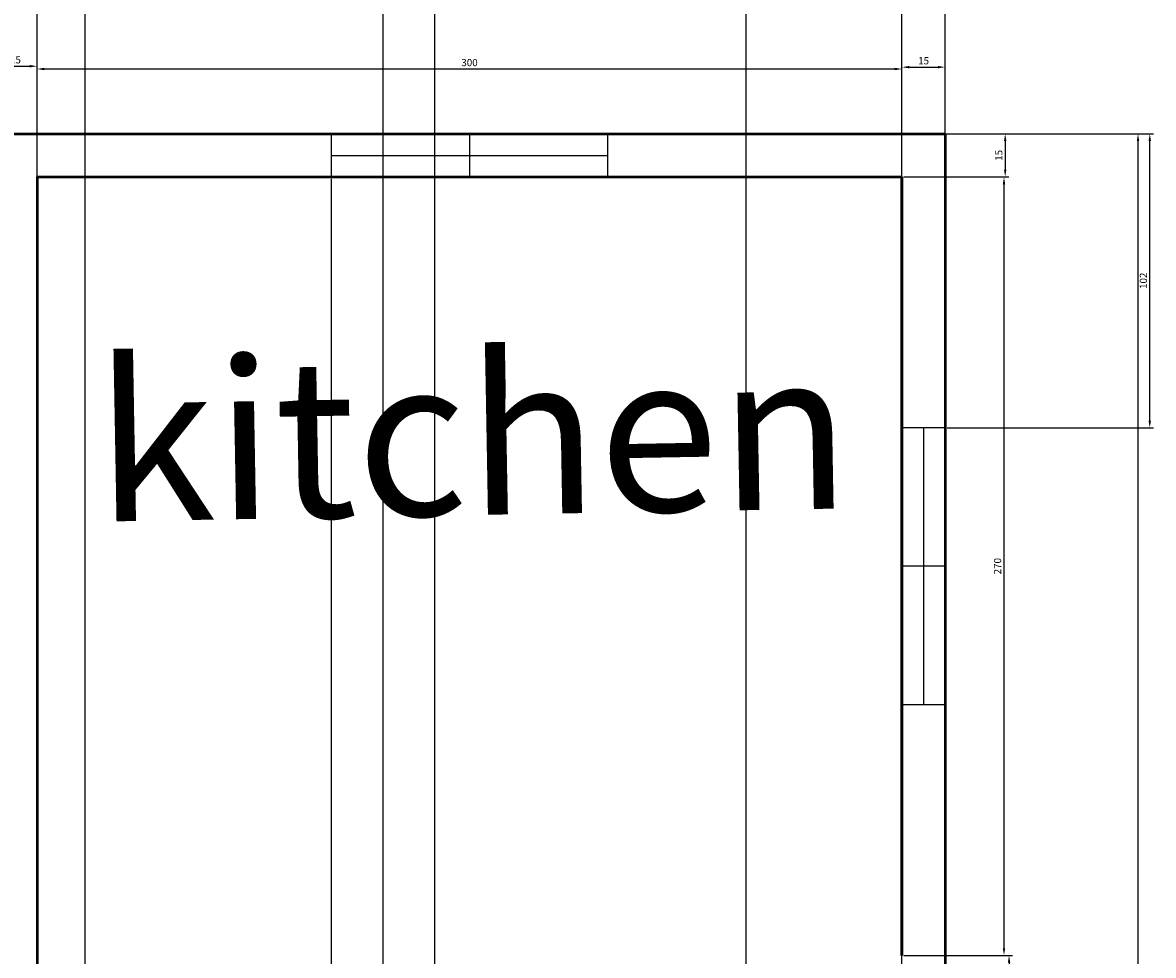
# Model space of a CAD drawing. Units: inches. Extents: x 604 to 3492, y -123 to 1737.
# Tile 10 of 20: x 1033 to 1425, y 1003 to 1326. Entities that reach past the tile are written whole.
import ezdxf

# ---------------------------------------------------------------- set-up
doc = ezdxf.new("R2010")
doc.units = ezdxf.units.IN
for name, color, linetype, lineweight in [('A-ANNO-DIMS', 2, 'Continuous', 18), ('A-AREA-IDEN', 7, 'Continuous', 25), ('A-GLAZ', 4, 'Continuous', 25), ('A-WALL', 7, 'Continuous', 50)]:
    doc.layers.add(name, color=color, linetype=linetype, lineweight=lineweight)
doc.styles.get("Standard").update_dxf_attribs({"font": 'arial.ttf'})
doc.dimstyles.new('ISO-25', dxfattribs={"dimtxt": 2.5, "dimasz": 2.5, "dimexe": 1.25, "dimexo": 0.625, "dimtad": 1, "dimtxsty": 'Standard', "dimcen": 2.5, "dimadec": 0, "dimazin": 0, "dimtfac": 1, "dimtmove": 0, "dimatfit": 3, "dimfxl": 1, "dimarcsym": 0})

# ---------------------------------------------------------------- blocks, each defined once
blk = doc.blocks.new('*D8')
at = {"layer": 'A-ANNO-DIMS', "color": 0, "lineweight": -2, "transparency": 16777216}
for p, q in [((1338.01, 1273.33), (1338.01, 1312.05)), ((1340.51, 1310.8), (1350.51, 1310.8)), ((1353.01, 1273.33), (1353.01, 1312.05))]:
    blk.add_line(p, q, dxfattribs=at)
at = {"layer": 'A-ANNO-DIMS', "color": 0, "transparency": 16777216}
for points in [[(1340.51, 1311.21), (1340.51, 1310.38), (1338.01, 1310.8)], [(1350.51, 1311.21), (1350.51, 1310.38), (1353.01, 1310.8)]]:
    blk.add_solid(points, dxfattribs=at)
at = {"layer": 'Defpoints', "color": 0, "transparency": 16777216}
for p in [(1353.01, 1310.8), (1338.01, 1272.7), (1353.01, 1272.7)]:
    blk.add_point(p, dxfattribs=at)
at = {"layer": 'A-ANNO-DIMS', "color": 0, "transparency": 16777216, "insert": (1345.51, 1312.7), "char_height": 2.5, "attachment_point": 5}
blk.add_mtext('15', dxfattribs=at)
blk = doc.blocks.new('*D9')
at = {"layer": 'A-ANNO-DIMS', "color": 0, "lineweight": -2, "transparency": 16777216}
for p, q in [((1038.01, 1273.33), (1038.01, 1311.41)), ((1040.51, 1310.16), (1335.51, 1310.16)), ((1338.01, 1273.33), (1338.01, 1311.41))]:
    blk.add_line(p, q, dxfattribs=at)
at = {"layer": 'A-ANNO-DIMS', "color": 0, "transparency": 16777216}
for points in [[(1040.51, 1310.58), (1040.51, 1309.74), (1038.01, 1310.16)], [(1335.51, 1310.58), (1335.51, 1309.74), (1338.01, 1310.16)]]:
    blk.add_solid(points, dxfattribs=at)
at = {"layer": 'Defpoints', "color": 0, "transparency": 16777216}
for p in [(1338.01, 1310.16), (1038.01, 1272.7), (1338.01, 1272.7)]:
    blk.add_point(p, dxfattribs=at)
at = {"layer": 'A-ANNO-DIMS', "color": 0, "transparency": 16777216, "insert": (1188.01, 1312.06), "char_height": 2.5, "attachment_point": 5}
blk.add_mtext('300', dxfattribs=at)
blk = doc.blocks.new('*D10')
at = {"layer": 'A-ANNO-DIMS', "color": 0, "lineweight": -2, "transparency": 16777216}
for p, q in [((1023.01, 1273.33), (1023.01, 1312.37)), ((1025.51, 1311.12), (1035.51, 1311.12)), ((1038.01, 1273.33), (1038.01, 1312.37))]:
    blk.add_line(p, q, dxfattribs=at)
at = {"layer": 'A-ANNO-DIMS', "color": 0, "transparency": 16777216}
for points in [[(1025.51, 1311.54), (1025.51, 1310.71), (1023.01, 1311.12)], [(1035.51, 1311.54), (1035.51, 1310.71), (1038.01, 1311.12)]]:
    blk.add_solid(points, dxfattribs=at)
at = {"layer": 'Defpoints', "color": 0, "transparency": 16777216}
for p in [(1038.01, 1311.12), (1023.01, 1272.7), (1038.01, 1272.7)]:
    blk.add_point(p, dxfattribs=at)
at = {"layer": 'A-ANNO-DIMS', "color": 0, "transparency": 16777216, "insert": (1030.51, 1313.02), "char_height": 2.5, "attachment_point": 5}
blk.add_mtext('15', dxfattribs=at)
blk = doc.blocks.new('*D13')
at = {"layer": 'A-ANNO-DIMS', "color": 0, "lineweight": -2, "transparency": 16777216}
for p, q in [((678.01, 1288.33), (678.01, 1383.12)), ((680.51, 1381.87), (1350.51, 1381.87)), ((1353.01, 1288.33), (1353.01, 1383.12))]:
    blk.add_line(p, q, dxfattribs=at)
at = {"layer": 'A-ANNO-DIMS', "color": 0, "transparency": 16777216}
for points in [[(680.51, 1382.29), (680.51, 1381.46), (678.01, 1381.87)], [(1350.51, 1382.29), (1350.51, 1381.46), (1353.01, 1381.87)]]:
    blk.add_solid(points, dxfattribs=at)
at = {"layer": 'Defpoints', "color": 0, "transparency": 16777216}
for p in [(1353.01, 1381.87), (678.01, 1287.7), (1353.01, 1287.7)]:
    blk.add_point(p, dxfattribs=at)
at = {"layer": 'A-ANNO-DIMS', "color": 0, "transparency": 16777216, "insert": (1015.51, 1383.78), "char_height": 2.5, "attachment_point": 5}
blk.add_mtext('675', dxfattribs=at)
blk = doc.blocks.new('*D14')
at = {"layer": 'A-ANNO-DIMS', "color": 0, "lineweight": -2, "transparency": 16777216}
for p, q in [((1338.64, 1287.7), (1375.06, 1287.7)), ((1373.81, 1285.2), (1373.81, 1275.2)), ((1338.64, 1272.7), (1375.06, 1272.7))]:
    blk.add_line(p, q, dxfattribs=at)
at = {"layer": 'A-ANNO-DIMS', "color": 0, "transparency": 16777216}
for points in [[(1373.4, 1285.2), (1374.23, 1285.2), (1373.81, 1287.7)], [(1373.4, 1275.2), (1374.23, 1275.2), (1373.81, 1272.7)]]:
    blk.add_solid(points, dxfattribs=at)
at = {"layer": 'Defpoints', "color": 0, "transparency": 16777216}
for p in [(1338.01, 1287.7), (1338.01, 1272.7), (1373.81, 1272.7)]:
    blk.add_point(p, dxfattribs=at)
at = {"layer": 'A-ANNO-DIMS', "color": 0, "transparency": 16777216, "insert": (1371.91, 1280.2), "char_height": 2.5, "attachment_point": 5, "rotation": 90}
blk.add_mtext('15', dxfattribs=at)
blk = doc.blocks.new('*D15')
at = {"layer": 'A-ANNO-DIMS', "color": 0, "lineweight": -2, "transparency": 16777216}
for p, q in [((1338.64, 1272.7), (1374.65, 1272.7)), ((1373.4, 1005.2), (1373.4, 1270.2)), ((1338.64, 1002.7), (1374.65, 1002.7))]:
    blk.add_line(p, q, dxfattribs=at)
at = {"layer": 'A-ANNO-DIMS', "color": 0, "transparency": 16777216}
for points in [[(1372.98, 1270.2), (1373.81, 1270.2), (1373.4, 1272.7)], [(1372.98, 1005.2), (1373.81, 1005.2), (1373.4, 1002.7)]]:
    blk.add_solid(points, dxfattribs=at)
at = {"layer": 'Defpoints', "color": 0, "transparency": 16777216}
for p in [(1338.01, 1272.7), (1373.4, 1272.7), (1338.01, 1002.7)]:
    blk.add_point(p, dxfattribs=at)
at = {"layer": 'A-ANNO-DIMS', "color": 0, "transparency": 16777216, "insert": (1371.49, 1137.7), "char_height": 2.5, "attachment_point": 5, "rotation": 90}
blk.add_mtext('270', dxfattribs=at)
blk = doc.blocks.new('*D16')
at = {"layer": 'A-ANNO-DIMS', "color": 0, "lineweight": -2, "transparency": 16777216}
for p, q in [((1338.64, 1002.7), (1376.4, 1002.7)), ((1375.15, 1000.2), (1375.15, 990.2)), ((1338.64, 987.7), (1376.4, 987.7))]:
    blk.add_line(p, q, dxfattribs=at)
at = {"layer": 'A-ANNO-DIMS', "color": 0, "transparency": 16777216}
for points in [[(1374.73, 1000.2), (1375.57, 1000.2), (1375.15, 1002.7)], [(1374.73, 990.2), (1375.57, 990.2), (1375.15, 987.7)]]:
    blk.add_solid(points, dxfattribs=at)
at = {"layer": 'Defpoints', "color": 0, "transparency": 16777216}
for p in [(1338.01, 1002.7), (1338.01, 987.7), (1375.15, 987.7)]:
    blk.add_point(p, dxfattribs=at)
at = {"layer": 'A-ANNO-DIMS', "color": 0, "transparency": 16777216, "insert": (1373.25, 995.2), "char_height": 2.5, "attachment_point": 5, "rotation": 90}
blk.add_mtext('15', dxfattribs=at)
blk = doc.blocks.new('*D20')
at = {"layer": 'A-ANNO-DIMS', "color": 0, "lineweight": -2, "transparency": 16777216}
for p, q in [((1353.64, 1287.7), (1421.14, 1287.7)), ((1419.89, 590.2), (1419.89, 1285.2)), ((1353.64, 587.7), (1421.14, 587.7))]:
    blk.add_line(p, q, dxfattribs=at)
at = {"layer": 'A-ANNO-DIMS', "color": 0, "transparency": 16777216}
for points in [[(1419.47, 1285.2), (1420.3, 1285.2), (1419.89, 1287.7)], [(1419.47, 590.2), (1420.3, 590.2), (1419.89, 587.7)]]:
    blk.add_solid(points, dxfattribs=at)
at = {"layer": 'Defpoints', "color": 0, "transparency": 16777216}
for p in [(1353.01, 1287.7), (1419.89, 1287.7), (1353.01, 587.7)]:
    blk.add_point(p, dxfattribs=at)
at = {"layer": 'A-ANNO-DIMS', "color": 0, "transparency": 16777216, "insert": (1417.98, 937.7), "char_height": 2.5, "attachment_point": 5, "rotation": 90}
blk.add_mtext('700', dxfattribs=at)
blk = doc.blocks.new('WIN-96')
for p, q in [((15, 96), (0, 96)), ((7.5, 96), (7.5, 0)), ((15, 96), (15, 0)), ((15, 48), (0, 48))]:
    blk.add_line(p, q)
blk.add_lwpolyline([(0, 96), (0, 0), (15, 0), (15, 96)], close=True)
blk = doc.blocks.new('*D86')
at = {"layer": 'A-ANNO-DIMS', "color": 0, "lineweight": -2, "transparency": 16777216}
for p, q in [((1038.01, 1272.08), (1038.01, 67.77)), ((1140.01, 1272.08), (1140.01, 67.77)), ((1040.51, 69.02), (1137.51, 69.02))]:
    blk.add_line(p, q, dxfattribs=at)
at = {"layer": 'A-ANNO-DIMS', "color": 0, "transparency": 16777216}
for points in [[(1040.51, 69.44), (1040.51, 68.61), (1038.01, 69.02)], [(1137.51, 69.44), (1137.51, 68.61), (1140.01, 69.02)]]:
    blk.add_solid(points, dxfattribs=at)
at = {"layer": 'Defpoints', "color": 0, "transparency": 16777216}
for p in [(1038.01, 1272.7), (1140.01, 1272.7), (1140.01, 69.02)]:
    blk.add_point(p, dxfattribs=at)
at = {"layer": 'A-ANNO-DIMS', "color": 0, "transparency": 16777216, "insert": (1089.01, 70.93), "char_height": 2.5, "attachment_point": 5}
blk.add_mtext('102', dxfattribs=at)
blk = doc.blocks.new('*D87')
at = {"layer": 'A-ANNO-DIMS', "color": 0, "lineweight": -2, "transparency": 16777216}
for p, q in [((1353.64, 1287.7), (1425.21, 1287.7)), ((1423.96, 1188.2), (1423.96, 1285.2)), ((1353.64, 1185.7), (1425.21, 1185.7))]:
    blk.add_line(p, q, dxfattribs=at)
at = {"layer": 'A-ANNO-DIMS', "color": 0, "transparency": 16777216}
for points in [[(1423.54, 1285.2), (1424.38, 1285.2), (1423.96, 1287.7)], [(1423.54, 1188.2), (1424.38, 1188.2), (1423.96, 1185.7)]]:
    blk.add_solid(points, dxfattribs=at)
at = {"layer": 'Defpoints', "color": 0, "transparency": 16777216}
for p in [(1353.01, 1287.7), (1423.96, 1287.7), (1353.01, 1185.7)]:
    blk.add_point(p, dxfattribs=at)
at = {"layer": 'A-ANNO-DIMS', "color": 0, "transparency": 16777216, "insert": (1422.06, 1236.7), "char_height": 2.5, "attachment_point": 5, "rotation": 90}
blk.add_mtext('102', dxfattribs=at)
blk = doc.blocks.new('*D93')
at = {"layer": 'A-ANNO-DIMS', "color": 0, "lineweight": -2, "transparency": 16777216}
for p, q in [((1038.01, 588.33), (1038.01, 1359.9)), ((1040.51, 1358.65), (1052.21, 1358.65)), ((1054.71, 588.27), (1054.71, 1359.9))]:
    blk.add_line(p, q, dxfattribs=at)
at = {"layer": 'A-ANNO-DIMS', "color": 0, "transparency": 16777216}
for points in [[(1040.51, 1359.07), (1040.51, 1358.23), (1038.01, 1358.65)], [(1052.21, 1359.07), (1052.21, 1358.23), (1054.71, 1358.65)]]:
    blk.add_solid(points, dxfattribs=at)
at = {"layer": 'Defpoints', "color": 0, "transparency": 16777216}
for p in [(1054.71, 1358.65), (1038.01, 587.7), (1054.71, 587.64)]:
    blk.add_point(p, dxfattribs=at)
at = {"layer": 'A-ANNO-DIMS', "color": 0, "transparency": 16777216, "insert": (1046.36, 1360.55), "char_height": 2.5, "attachment_point": 5}
blk.add_mtext('16.697', dxfattribs=at)
blk = doc.blocks.new('*D95')
at = {"layer": 'A-ANNO-DIMS', "color": 0, "lineweight": -2, "transparency": 16777216}
for p, q in [((1284.01, 740.33), (1284.01, 1359.9)), ((1286.51, 1358.65), (1335.51, 1358.65)), ((1338.01, 740.33), (1338.01, 1359.9))]:
    blk.add_line(p, q, dxfattribs=at)
at = {"layer": 'A-ANNO-DIMS', "color": 0, "transparency": 16777216}
for points in [[(1286.51, 1359.07), (1286.51, 1358.23), (1284.01, 1358.65)], [(1335.51, 1359.07), (1335.51, 1358.23), (1338.01, 1358.65)]]:
    blk.add_solid(points, dxfattribs=at)
at = {"layer": 'Defpoints', "color": 0, "transparency": 16777216}
for p in [(1338.01, 1358.65), (1284.01, 739.7), (1338.01, 739.7)]:
    blk.add_point(p, dxfattribs=at)
at = {"layer": 'A-ANNO-DIMS', "color": 0, "transparency": 16777216, "insert": (1311.01, 1360.55), "char_height": 2.5, "attachment_point": 5}
blk.add_mtext('54', dxfattribs=at)
blk = doc.blocks.new('*D96')
at = {"layer": 'A-ANNO-DIMS', "color": 0, "lineweight": -2, "transparency": 16777216}
for p, q in [((1158.01, 740.33), (1158.01, 1359.9)), ((1160.51, 1358.65), (1173.51, 1358.65)), ((1176.01, 740.33), (1176.01, 1359.9))]:
    blk.add_line(p, q, dxfattribs=at)
at = {"layer": 'A-ANNO-DIMS', "color": 0, "transparency": 16777216}
for points in [[(1160.51, 1359.07), (1160.51, 1358.23), (1158.01, 1358.65)], [(1173.51, 1359.07), (1173.51, 1358.23), (1176.01, 1358.65)]]:
    blk.add_solid(points, dxfattribs=at)
at = {"layer": 'Defpoints', "color": 0, "transparency": 16777216}
for p in [(1176.01, 1358.65), (1158.01, 739.7), (1176.01, 739.7)]:
    blk.add_point(p, dxfattribs=at)
at = {"layer": 'A-ANNO-DIMS', "color": 0, "transparency": 16777216, "insert": (1167.01, 1360.55), "char_height": 2.5, "attachment_point": 5}
blk.add_mtext('18', dxfattribs=at)

msp = doc.modelspace()

# ---------------------------------------------------------------- linework, layer by layer
at = {"layer": 'A-WALL'}
for p, q in [((678.0111, 1287.7004), (1353.0111, 1287.7004)), ((1038.0111, 1287.7004), (1338.0111, 1287.7004)), ((1353.0111, 1287.7004), (1353.0111, 587.7004)), ((1038.0111, 1272.7004), (1038.0111, 897.7004)), ((1038.0111, 1272.7004), (1338.0111, 1272.7004)), ((1038.0111, 1272.7004), (1338.0111, 1272.7004)), ((1338.0111, 1272.7004), (1338.0111, 1002.7004)), ((1338.0111, 1002.7004), (1338.0111, 1272.7004))]:
    msp.add_line(p, q, dxfattribs=at)

# ---------------------------------------------------------------- block references
at = {"layer": 'A-GLAZ', "rotation": 89.99999999999905}
msp.add_blockref('WIN-96', (1236.0111, 1272.7004), dxfattribs=at)
at = {"layer": 'A-GLAZ'}
msp.add_blockref('WIN-96', (1338.0111, 1089.7004), dxfattribs=at)

# ---------------------------------------------------------------- texts
at = {"layer": 'A-AREA-IDEN'}
msp.add_text('kitchen', height=55.10325, rotation=1.013147, dxfattribs=at).set_placement((1058.6651, 1153.1386))

# ---------------------------------------------------------------- dimensions: what is measured, and where the dimension line sits
at = {"layer": 'A-ANNO-DIMS'}
for base, p1, p2, override, picture, middle in [((1353.0111, 1381.8744), (678.0111, 1287.7004), (1353.0111, 1287.7004), {"dimclrd": 0, "dimclre": 0, "dimclrt": 0}, '*D13', (1015.5111, 1383.7759)), ((1054.7083, 1358.6504), (1038.0111, 587.7004), (1054.7083, 587.6435), {"dimdec": 3, "dimlfac": 1, "dimrnd": 0, "dimzin": 0, "dimdsep": 46, "dimlunit": 2}, '*D93', (1046.3597, 1360.5519)), ((1176.0111, 1358.6504), (1158.0111, 739.7004), (1176.0111, 739.7004), {"dimdec": 0, "dimlfac": 1, "dimrnd": 0, "dimzin": 0, "dimdsep": 46, "dimlunit": 2}, '*D96', (1167.0111, 1360.5519)), ((1338.0111, 1358.6504), (1284.0111, 739.7004), (1338.0111, 739.7004), {"dimdec": 0, "dimlfac": 1, "dimrnd": 0, "dimzin": 0, "dimdsep": 46, "dimlunit": 2}, '*D95', (1311.0111, 1360.5468)), ((1038.0111, 1311.1217), (1023.0111, 1272.7004), (1038.0111, 1272.7004), {"dimclrd": 0, "dimclre": 0, "dimclrt": 0}, '*D10', (1030.5111, 1313.0232)), ((1353.0111, 1310.7965), (1338.0111, 1272.7004), (1353.0111, 1272.7004), {"dimclrd": 0, "dimclre": 0, "dimclrt": 0}, '*D8', (1345.5111, 1312.6979)), ((1338.0111, 1310.1605), (1038.0111, 1272.7004), (1338.0111, 1272.7004), {"dimclrd": 0, "dimclre": 0, "dimclrt": 0}, '*D9', (1188.0111, 1312.0628)), ((1140.0111, 69.0242), (1038.0111, 1272.7004), (1140.0111, 1272.7004), {"dimdec": 0, "dimlfac": 1, "dimrnd": 0, "dimzin": 0, "dimdsep": 46, "dimlunit": 2}, '*D86', (1089.0111, 70.9256))]:
    dim = msp.add_linear_dim(base=base, p1=p1, p2=p2, dimstyle='ISO-25', override=override, dxfattribs=at)
    dim.commit()
    dim.dimension.update_dxf_attribs({"geometry": picture, "text_midpoint": middle})
for base, p1, p2, override, picture, middle in [((1373.8127, 1272.7004), (1338.0111, 1287.7004), (1338.0111, 1272.7004), {"dimclrd": 0, "dimclre": 0, "dimclrt": 0}, '*D14', (1371.9113, 1280.2004)), ((1419.8851, 1287.7004), (1353.0111, 587.7004), (1353.0111, 1287.7004), {"dimclrd": 0, "dimclre": 0, "dimclrt": 0}, '*D20', (1417.9836, 937.7004)), ((1423.9611, 1287.7004), (1353.0111, 1185.7004), (1353.0111, 1287.7004), {"dimdec": 0, "dimlfac": 1, "dimrnd": 0, "dimzin": 0, "dimdsep": 46, "dimlunit": 2}, '*D87', (1422.0597, 1236.7004)), ((1375.1487, 987.7004), (1338.0111, 1002.7004), (1338.0111, 987.7004), {"dimclrd": 0, "dimclre": 0, "dimclrt": 0}, '*D16', (1373.2472, 995.2004))]:
    dim = msp.add_linear_dim(base=base, p1=p1, p2=p2, angle=90, dimstyle='ISO-25', override=override, dxfattribs=at)
    dim.commit()
    dim.dimension.update_dxf_attribs({"geometry": picture, "text_midpoint": middle})
dim = msp.add_aligned_dim(p1=(1338.0111, 1002.7004), p2=(1338.0111, 1272.7004), distance=-35.3849, dimstyle='ISO-25', override={"dimclrd": 0, "dimclre": 0, "dimclrt": 0}, dxfattribs=at)
dim.commit()
dim.dimension.update_dxf_attribs({"geometry": '*D15', "text_midpoint": (1371.4946, 1137.7004)})

doc.saveas('drawing.dxf')
